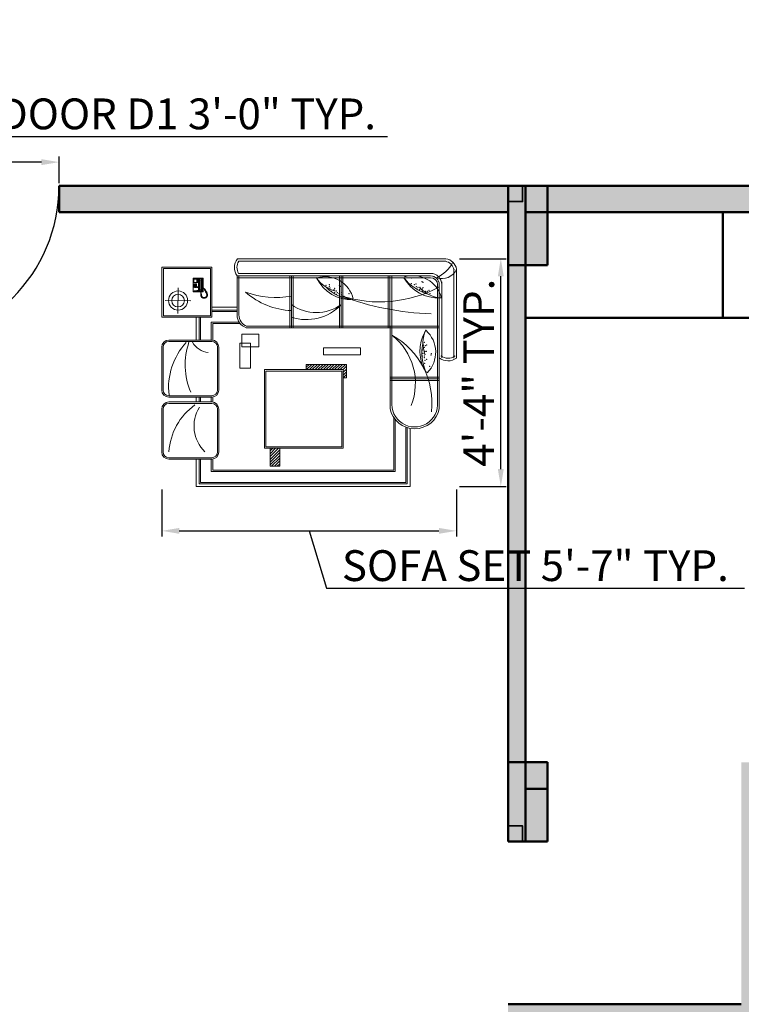
# Model space of a CAD drawing. Units: inches. Extents: x -7 to 1228, y -146 to 1091.
# Tile 24 of 88: x 269 to 433, y 307 to 531. Entities that reach past the tile are written whole.
import ezdxf

# ---------------------------------------------------------------- set-up
doc = ezdxf.new("R2010")
doc.units = ezdxf.units.IN
for name, color, linetype, lineweight in [('A-ANNO-DIMS', 2, 'Continuous', 18), ('A-COLS', 6, 'Continuous', 35), ('A-DOOR', 4, 'Continuous', 25), ('A-FURN', 8, 'Continuous', 18), ('A-WALL', 7, 'Continuous', 50), ('A-WALL-PATT', 251, 'Continuous', 13)]:
    doc.layers.add(name, color=color, linetype=linetype, lineweight=lineweight)
doc.styles.get("Standard").update_dxf_attribs({"font": 'arial.ttf'})
doc.dimstyles.new('ISO-25', dxfattribs={"dimtxt": 7, "dimasz": 4, "dimexe": 1.25, "dimexo": 0.625, "dimtad": 1, "dimdec": 1, "dimlunit": 3, "dimtxsty": 'Standard', "dimcen": 2.5, "dimadec": 0, "dimazin": 0, "dimtfac": 1, "dimtdec": 1, "dimtmove": 1, "dimatfit": 3, "dimfxl": 1, "dimarcsym": 0})

# ---------------------------------------------------------------- blocks, each defined once
blk = doc.blocks.new('A$C327A19D4')
for p, q in [((1059, 3191), (3976, 3191)), ((703, 3073), (3, 3073)), ((3, 3073), (3, 2373)), ((683, 3053), (23, 3053)), ((23, 3053), (23, 2393)), ((683, 2393), (683, 3053)), ((703, 2373), (703, 3073)), ((1078, 3155), (3976, 3155)), ((4090, 3043), (4090, 1800)), ((4126, 3043), (4126, 1800)), ((1056, 2949), (3763, 2949)), ((1056, 2403), (1056, 2949)), ((1056, 2925), (3763, 2925)), ((1076, 2985), (3780, 2985)), ((1080, 2403), (1080, 2949)), ((1791, 2223), (1791, 2949)), ((1815, 2465), (1815, 2949)), ((1839, 2223), (1839, 2949)), ((2487, 2223), (2487, 2949)), ((2511, 2223), (2511, 2949)), ((2535, 2223), (2535, 2949)), ((3169, 2223), (3169, 2949)), ((3193, 2465), (3193, 2949)), ((3221, 1195), (3221, 2949)), ((231, 2784), (227, 2425)), ((1815, 2223), (1815, 2872)), ((1815, 2223), (1815, 2872)), ((1815, 2465), (1815, 2872)), ((1815, 2465), (1815, 2872)), ((3193, 2223), (3193, 2872)), ((3193, 2223), (3193, 2872)), ((3193, 2465), (3193, 2872)), ((3193, 2465), (3193, 2872)), ((3860, 2828), (3860, 1185)), ((3884, 2828), (3884, 1095)), ((3920, 2867), (3920, 1802)), ((49, 2607), (409, 2603)), ((703, 2512), (1056, 2512)), ((3, 2373), (703, 2373)), ((23, 2393), (683, 2393)), ((484, 2052), (484, 2373)), ((524, 2052), (524, 2373)), ((544, 2052), (544, 2373)), ((703, 2472), (1056, 2472)), ((703, 2452), (1056, 2452)), ((694, 2052), (694, 2302)), ((694, 2302), (1084, 2302)), ((714, 2051), (714, 2282)), ((714, 2282), (1098, 2282)), ((3884, 2247), (1184, 2247)), ((3884, 2223), (1184, 2223)), ((3195, 2235), (3195, 1095)), ((1119, 2135), (1357, 2135)), ((1119, 1958), (1119, 2135)), ((1357, 2135), (1357, 1958)), ((1092, 2007), (1244, 2007)), ((1092, 1659), (1092, 2007)), ((1357, 1958), (1119, 1958)), ((1244, 2007), (1244, 1659)), ((2265, 1945), (2780, 1945)), ((2265, 1845), (2265, 1945)), ((2780, 1945), (2780, 1845)), ((2780, 1845), (2265, 1845)), ((1244, 1659), (1092, 1659)), ((2023, 1638), (2023, 1711)), ((2023, 1711), (2585, 1711)), ((2585, 1711), (2585, 1522)), ((2539, 1638), (1439, 1638)), ((1439, 1638), (1439, 538)), ((2519, 1618), (1459, 1618)), ((1459, 1618), (1459, 558)), ((2519, 558), (2519, 1618)), ((2539, 538), (2539, 1638)), ((2585, 1522), (2539, 1522)), ((3884, 1532), (3195, 1532)), ((3884, 1508), (3195, 1508)), ((3884, 1484), (3195, 1484)), ((484, 1185), (484, 1252)), ((524, 1185), (524, 1252)), ((544, 1185), (544, 1252)), ((694, 1185), (694, 1252)), ((714, 1184), (714, 1253)), ((3247, 967), (3247, 230)), ((3267, 940), (3267, 210)), ((3417, 832), (3417, 60)), ((3437, 825), (3437, 40)), ((3477, 816), (3477, 0)), ((1459, 558), (2519, 558)), ((1439, 538), (2539, 538)), ((1516, 538), (1651, 538)), ((1516, 285), (1516, 538)), ((1651, 538), (1651, 285)), ((484, 0), (484, 385)), ((524, 40), (524, 385)), ((544, 60), (544, 385)), ((694, 210), (694, 385)), ((714, 230), (714, 386)), ((1651, 285), (1516, 285)), ((3267, 210), (694, 210)), ((3247, 230), (714, 230)), ((3437, 40), (524, 40)), ((3417, 60), (544, 60)), ((3477, 0), (484, 0))]:
    blk.add_line(p, q)
at = {"linetype": 'ByBlock'}
for p, q in [((438, 2915), (440, 2918)), ((439, 2728), (438, 2915)), ((440, 2918), (576, 2919)), ((451, 2906), (490, 2906)), ((451, 2856), (451, 2906)), ((490, 2906), (491, 2856)), ((505, 2903), (494, 2903)), ((494, 2903), (494, 2899)), ((494, 2899), (505, 2899)), ((495, 2895), (495, 2891)), ((505, 2895), (495, 2895)), ((505, 2899), (505, 2903)), ((505, 2891), (505, 2895)), ((515, 2908), (520, 2914)), ((516, 2744), (515, 2908)), ((520, 2910), (519, 2905)), ((519, 2905), (531, 2893)), ((519, 2905), (519, 2868)), ((520, 2914), (561, 2915)), ((526, 2913), (520, 2910)), ((532, 2895), (526, 2913)), ((526, 2913), (558, 2913)), ((531, 2893), (532, 2895)), ((551, 2896), (532, 2895)), ((551, 2896), (558, 2913)), ((553, 2893), (551, 2896)), ((565, 2905), (553, 2893)), ((558, 2913), (563, 2911)), ((561, 2915), (568, 2908)), ((563, 2911), (565, 2905)), ((565, 2905), (565, 2869)), ((568, 2908), (569, 2745)), ((576, 2919), (578, 2916)), ((578, 2916), (580, 2729)), ((491, 2856), (451, 2856)), ((453, 2831), (453, 2839)), ((453, 2839), (461, 2839)), ((461, 2831), (453, 2831)), ((453, 2824), (461, 2825)), ((453, 2816), (453, 2824)), ((461, 2816), (453, 2816)), ((453, 2801), (453, 2810)), ((453, 2810), (461, 2810)), ((461, 2802), (453, 2801)), ((453, 2787), (453, 2795)), ((453, 2795), (461, 2795)), ((461, 2787), (453, 2787)), ((461, 2839), (461, 2831)), ((461, 2825), (461, 2816)), ((461, 2810), (461, 2802)), ((461, 2795), (461, 2787)), ((466, 2839), (475, 2840)), ((467, 2831), (466, 2839)), ((475, 2831), (467, 2831)), ((467, 2816), (467, 2825)), ((467, 2825), (475, 2825)), ((475, 2817), (467, 2816)), ((467, 2802), (467, 2810)), ((467, 2810), (475, 2810)), ((475, 2802), (467, 2802)), ((467, 2787), (467, 2795)), ((467, 2795), (475, 2795)), ((475, 2787), (467, 2787)), ((475, 2840), (475, 2831)), ((475, 2825), (475, 2817)), ((475, 2810), (475, 2802)), ((475, 2795), (475, 2787)), ((480, 2840), (488, 2840)), ((480, 2831), (480, 2840)), ((488, 2832), (480, 2831)), ((480, 2817), (480, 2825)), ((480, 2825), (488, 2825)), ((488, 2817), (480, 2817)), ((480, 2810), (488, 2810)), ((480, 2802), (480, 2810)), ((488, 2802), (480, 2802)), ((480, 2787), (480, 2795)), ((480, 2795), (488, 2795)), ((488, 2787), (480, 2787)), ((488, 2840), (488, 2832)), ((488, 2825), (488, 2817)), ((488, 2810), (488, 2802)), ((488, 2795), (488, 2787)), ((495, 2891), (505, 2891)), ((495, 2887), (495, 2883)), ((505, 2887), (495, 2887)), ((495, 2883), (505, 2883)), ((495, 2879), (495, 2875)), ((505, 2879), (495, 2879)), ((495, 2875), (505, 2875)), ((495, 2871), (495, 2867)), ((506, 2871), (495, 2871)), ((495, 2867), (506, 2867)), ((495, 2863), (495, 2859)), ((506, 2863), (495, 2863)), ((495, 2859), (506, 2859)), ((497, 2795), (507, 2795)), ((497, 2787), (497, 2795)), ((507, 2787), (497, 2787)), ((505, 2883), (505, 2887)), ((505, 2875), (505, 2879)), ((506, 2867), (506, 2871)), ((506, 2859), (506, 2863)), ((507, 2795), (507, 2787)), ((519, 2868), (522, 2862)), ((520, 2783), (522, 2790)), ((520, 2746), (520, 2783)), ((520, 2746), (532, 2759)), ((522, 2862), (526, 2855)), ((522, 2790), (526, 2797)), ((526, 2855), (527, 2845)), ((526, 2797), (528, 2806)), ((527, 2845), (527, 2832)), ((528, 2806), (527, 2832)), ((532, 2832), (531, 2893)), ((532, 2832), (532, 2759)), ((532, 2759), (533, 2756)), ((554, 2759), (552, 2756)), ((553, 2832), (553, 2893)), ((553, 2832), (554, 2759)), ((566, 2747), (554, 2759)), ((558, 2855), (557, 2846)), ((557, 2846), (557, 2832)), ((557, 2806), (557, 2832)), ((559, 2797), (557, 2806)), ((562, 2862), (558, 2855)), ((563, 2790), (559, 2797)), ((565, 2869), (562, 2862)), ((566, 2783), (563, 2790)), ((566, 2747), (566, 2783)), ((587, 2779), (579, 2779)), ((579, 2775), (584, 2774)), ((584, 2774), (587, 2772)), ((590, 2777), (587, 2779)), ((587, 2772), (591, 2770)), ((594, 2771), (590, 2777)), ((591, 2770), (593, 2768)), ((595, 2768), (592, 2765)), ((592, 2765), (597, 2757)), ((593, 2768), (595, 2768)), ((599, 2771), (594, 2771)), ((597, 2757), (606, 2742)), ((602, 2770), (599, 2771)), ((599, 2760), (603, 2767)), ((606, 2763), (599, 2760)), ((603, 2767), (602, 2770)), ((604, 2750), (608, 2758)), ((608, 2758), (606, 2763)), ((442, 2726), (439, 2728)), ((543, 2726), (442, 2726)), ((468, 2743), (455, 2743)), ((455, 2743), (455, 2735)), ((455, 2735), (469, 2735)), ((469, 2735), (468, 2743)), ((487, 2743), (474, 2743)), ((474, 2743), (474, 2735)), ((474, 2735), (487, 2735)), ((487, 2735), (487, 2743)), ((493, 2744), (493, 2735)), ((506, 2744), (493, 2744)), ((493, 2735), (506, 2735)), ((506, 2735), (506, 2744)), ((523, 2737), (516, 2744)), ((521, 2741), (520, 2746)), ((527, 2738), (521, 2741)), ((542, 2737), (523, 2737)), ((533, 2756), (527, 2738)), ((527, 2738), (542, 2738)), ((552, 2756), (533, 2756)), ((546, 2743), (542, 2743)), ((542, 2743), (542, 2731)), ((542, 2731), (545, 2717)), ((545, 2717), (549, 2704)), ((547, 2732), (546, 2743)), ((546, 2738), (559, 2739)), ((562, 2737), (546, 2737)), ((549, 2696), (546, 2692)), ((546, 2692), (546, 2686)), ((546, 2686), (554, 2685)), ((554, 2685), (546, 2680)), ((546, 2680), (547, 2672)), ((548, 2723), (547, 2732)), ((547, 2672), (555, 2672)), ((577, 2726), (548, 2726)), ((552, 2710), (548, 2723)), ((549, 2704), (548, 2697)), ((548, 2697), (549, 2696)), ((555, 2672), (548, 2666)), ((548, 2666), (551, 2659)), ((551, 2659), (560, 2661)), ((552, 2756), (559, 2739)), ((553, 2703), (552, 2710)), ((552, 2696), (553, 2703)), ((557, 2693), (552, 2696)), ((556, 2687), (557, 2693)), ((558, 2669), (556, 2687)), ((560, 2661), (556, 2653)), ((556, 2653), (560, 2648)), ((568, 2656), (558, 2669)), ((559, 2739), (565, 2741)), ((560, 2648), (566, 2653)), ((569, 2745), (562, 2737)), ((565, 2741), (566, 2747)), ((566, 2653), (565, 2646)), ((565, 2646), (570, 2642)), ((583, 2649), (568, 2656)), ((570, 2642), (577, 2648)), ((577, 2648), (576, 2639)), ((576, 2639), (582, 2637)), ((580, 2729), (577, 2726)), ((582, 2637), (585, 2645)), ((599, 2647), (583, 2649)), ((585, 2645), (589, 2637)), ((589, 2637), (593, 2637)), ((593, 2637), (595, 2645)), ((595, 2645), (598, 2636)), ((598, 2636), (604, 2637)), ((615, 2654), (599, 2647)), ((612, 2753), (604, 2750)), ((604, 2645), (610, 2639)), ((604, 2637), (604, 2645)), ((606, 2742), (612, 2731)), ((608, 2742), (614, 2749)), ((615, 2746), (608, 2742)), ((610, 2639), (615, 2642)), ((614, 2749), (612, 2753)), ((612, 2731), (614, 2730)), ((613, 2733), (618, 2740)), ((621, 2736), (613, 2733)), ((614, 2730), (613, 2728)), ((613, 2728), (622, 2712)), ((614, 2650), (619, 2643)), ((615, 2642), (614, 2650)), ((618, 2740), (615, 2746)), ((627, 2666), (615, 2654)), ((619, 2643), (624, 2647)), ((620, 2723), (624, 2730)), ((627, 2725), (620, 2723)), ((620, 2654), (628, 2651)), ((624, 2647), (620, 2654)), ((624, 2730), (621, 2736)), ((622, 2712), (631, 2687)), ((626, 2712), (630, 2720)), ((634, 2713), (626, 2712)), ((630, 2720), (627, 2725)), ((631, 2687), (627, 2666)), ((628, 2702), (636, 2705)), ((637, 2702), (628, 2702)), ((628, 2661), (636, 2659)), ((632, 2654), (628, 2661)), ((628, 2651), (632, 2654)), ((631, 2672), (640, 2672)), ((638, 2665), (631, 2672)), ((633, 2691), (639, 2696)), ((641, 2691), (633, 2691)), ((636, 2705), (634, 2713)), ((634, 2681), (642, 2684)), ((641, 2677), (634, 2681)), ((636, 2659), (638, 2665)), ((639, 2696), (637, 2702)), ((640, 2672), (641, 2677)), ((642, 2684), (641, 2691))]:
    blk.add_line(p, q, dxfattribs=at)
at = {"ltscale": 5}
for p, q in [((0, 1352), (0, 1952)), ((20, 1352), (20, 1952)), ((100, 2052), (700, 2052)), ((100, 2032), (700, 2032)), ((780, 1952), (780, 1352)), ((800, 1952), (800, 1352)), ((2023, 1673), (2061, 1711)), ((2027, 1638), (2100, 1711)), ((2067, 1638), (2139, 1711)), ((2106, 1638), (2179, 1711)), ((2145, 1638), (2218, 1711)), ((2184, 1638), (2257, 1711)), ((2224, 1638), (2296, 1711)), ((2263, 1638), (2336, 1711)), ((2302, 1638), (2375, 1711)), ((2341, 1638), (2414, 1711)), ((2381, 1638), (2453, 1711)), ((2420, 1638), (2493, 1711)), ((2459, 1638), (2532, 1711)), ((2498, 1638), (2571, 1711)), ((2538, 1638), (2585, 1685)), ((2539, 1601), (2585, 1646)), ((2539, 1561), (2585, 1607)), ((2539, 1522), (2585, 1568)), ((2578, 1522), (2585, 1528)), ((700, 1272), (100, 1272)), ((700, 1252), (100, 1252)), ((100, 1185), (700, 1185)), ((100, 1165), (700, 1165)), ((0, 485), (0, 1085)), ((20, 485), (20, 1085)), ((780, 1085), (780, 485)), ((800, 1085), (800, 485)), ((1516, 499), (1555, 538)), ((1516, 460), (1594, 538)), ((1516, 421), (1634, 538)), ((1516, 382), (1651, 516)), ((1516, 342), (1651, 477)), ((1516, 303), (1651, 438)), ((700, 405), (100, 405)), ((700, 385), (100, 385)), ((1537, 285), (1651, 398)), ((1576, 285), (1651, 359)), ((1616, 285), (1651, 320))]:
    blk.add_line(p, q, dxfattribs=at)
for radius in [134, 88.7]:
    blk.add_circle((229, 2605), radius)
for centre, radius, start, end in [((1218, 3068), 201, 142.4201, 216.3682), ((3943, 3007), 187, 10.9855, 79.893), ((1218, 3068), 165, 148.4003, 210.2229), ((3657, 3353), 468, 293.6733, 332.9672), ((3921, 3138), 226, 250.4844, 335.1673), ((3943, 3007), 150, 10.9855, 79.893), ((2545, 3192), 468, 214.7097, 257.8799), ((2283, 2531), 409, 13.4523, 105.9639), ((2657, 3163), 547, 207.1715, 271.8037), ((3869, 3188), 547, 208.8478, 273.48), ((3911, 3323), 657, 217.6007, 253.5739), ((3517, 2544), 409, 14.6876, 107.1992), ((3763, 2828), 157, 0, 90), ((3763, 2828), 121, 0, 90), ((3763, 2828), 96.8, 0, 90), ((2752, 3267), 657, 227.0776, 263.0508), ((3052, 4350), 1764, 252.1519, 298.1592), ((3951, 3106), 468, 222.7716, 265.9418), ((1594, 3859), 1211, 249.7283, 280.5443), ((1853, 3485), 1021, 228.2765, 267.8541), ((3865, 6197), 3777, 248.9971, 268.5461), ((2024, 3008), 670, 251.8392, 316.629), ((2163, 3036), 599, 234.5154, 305.4846), ((1243, 2401), 187, 179.2584, 251.6848), ((1243, 2401), 163, 179.2584, 251.6848), ((4159, 1898), 547, 149.1529, 213.7851), ((4124, 2008), 468, 156.691, 199.8613), ((3425, 1881), 409, 315.4337, 47.9453), ((4298, 1873), 657, 169.059, 205.0321), ((4007, 1962), 201, 232.4201, 306.3682), ((4007, 1962), 165, 232.4201, 306.3682)]:
    blk.add_arc(centre, radius, start, end)
at = {"ltscale": 20}
for centre, radius, start, end in [((2701, 1449), 849, 338.2682, 52.2695), ((2703, 1175), 1078, 353.1988, 61.2564), ((3540, 1156), 321, 172.9078, 5.2194), ((3540, 1161), 351, 190.8398, 349.1602)]:
    blk.add_arc(centre, radius, start, end, dxfattribs=at)
at = {"ltscale": 5}
for centre, radius, start, end in [((100, 1952), 100, 90, 180), ((100, 1952), 80, 90, 180), ((1024, 1388), 928, 137.1341, 186.5635), ((1307, 1706), 979, 160.9364, 203.1944), ((676, 2156), 279, 209.1633, 264.4137), ((700, 1952), 100, 0, 90), ((700, 1952), 80, 0, 90), ((100, 1352), 100, 180, 270), ((100, 1352), 80, 180, 270), ((700, 1352), 80, 270, 0), ((700, 1352), 100, 270, 0), ((100, 1085), 100, 90, 180), ((100, 1085), 80, 90, 180), ((968, 436), 868, 125.4807, 176.5616), ((949, 846), 497, 147.8484, 226.1244), ((700, 1085), 100, 0, 90), ((700, 1085), 80, 0, 90), ((100, 485), 100, 180, 270), ((100, 485), 80, 180, 270), ((700, 485), 100, 270, 0), ((700, 485), 80, 270, 0)]:
    blk.add_arc(centre, radius, start, end, dxfattribs=at)
for p in [(3492, 2920), (2298, 2818), (2329, 2780), (2344, 2802), (2345, 2825), (2356, 2781), (2410, 2757), (2421, 2774), (2485, 2814), (2498, 2803), (3495, 2842), (3535, 2825), (3560, 2838), (3561, 2800), (3571, 2765), (3585, 2789), (3609, 2758), (3612, 2788), (3641, 2868), (3647, 2768), (3655, 2787), (3657, 2862), (2375, 2736), (2421, 2720), (2444, 2738), (2445, 2691), (2459, 2715), (2481, 2700), (2514, 2718), (2515, 2690), (2551, 2664), (2620, 2701), (3646, 2728), (3694, 2735), (3707, 2710), (3719, 2734), (3738, 2747), (3756, 2703), (3660, 1974), (3676, 1951), (3677, 2020), (3687, 1973), (3707, 1984), (3646, 1828), (3648, 1911), (3658, 1864), (3673, 1803), (3674, 1829), (3684, 1893), (3686, 1853), (3705, 1892), (3770, 1842), (3772, 1859), (3680, 1724), (3683, 1768), (3706, 1784), (3748, 1685)]:
    blk.add_point(p)
blk = doc.blocks.new('DOOR-900')
blk.add_line((36, 0), (36, 36))
blk.add_arc((36, 0), 36, 90, 180)
blk = doc.blocks.new('*D40')
at = {"layer": 'A-ANNO-DIMS', "color": 0, "lineweight": -2, "transparency": 16777216}
for p, q in [((301.32, 424.02), (301.32, 413.35)), ((368.31, 424.02), (368.31, 413.35)), ((305.32, 414.6), (364.31, 414.6)), ((334.82, 414.6), (338.73, 401.55)), ((338.73, 401.55), (433.69, 401.55))]:
    blk.add_line(p, q, dxfattribs=at)
at = {"layer": 'A-ANNO-DIMS', "color": 0, "transparency": 16777216}
for points in [[(305.32, 415.26), (305.32, 413.93), (301.32, 414.6)], [(364.31, 415.26), (364.31, 413.93), (368.31, 414.6)]]:
    blk.add_solid(points, dxfattribs=at)
at = {"layer": 'Defpoints', "color": 0, "transparency": 16777216}
for p in [(301.32, 424.65), (368.31, 424.65), (368.31, 414.6)]:
    blk.add_point(p, dxfattribs=at)
at = {"layer": 'A-ANNO-DIMS', "color": 0, "transparency": 16777216, "insert": (386.21, 405.79), "char_height": 7, "attachment_point": 5}
blk.add_mtext('SOFA SET 5\'-7" TYP.', dxfattribs=at)
blk = doc.blocks.new('*D41')
at = {"layer": 'A-ANNO-DIMS', "color": 0, "lineweight": -2, "transparency": 16777216}
for p, q in [((368.94, 476.46), (379.61, 476.46)), ((378.36, 428.65), (378.36, 472.46)), ((368.94, 424.65), (379.61, 424.65))]:
    blk.add_line(p, q, dxfattribs=at)
at = {"layer": 'A-ANNO-DIMS', "color": 0, "transparency": 16777216}
for points in [[(377.69, 472.46), (379.03, 472.46), (378.36, 476.46)], [(377.69, 428.65), (379.03, 428.65), (378.36, 424.65)]]:
    blk.add_solid(points, dxfattribs=at)
at = {"layer": 'Defpoints', "color": 0, "transparency": 16777216}
for p in [(368.31, 476.46), (378.36, 476.46), (368.31, 424.65)]:
    blk.add_point(p, dxfattribs=at)
at = {"layer": 'A-ANNO-DIMS', "color": 0, "transparency": 16777216, "insert": (374.23, 450.55), "char_height": 7, "attachment_point": 5, "rotation": 90}
blk.add_mtext('4\'-4" TYP.', dxfattribs=at)
blk = doc.blocks.new('*D44')
at = {"layer": 'A-ANNO-DIMS', "color": 0, "lineweight": -2, "transparency": 16777216}
for p, q in [((260, 498.4), (261.74, 504.21)), ((261.74, 504.21), (352.58, 504.21)), ((242, 493.62), (242, 499.65)), ((278, 493.62), (278, 499.65)), ((274, 498.4), (246, 498.4))]:
    blk.add_line(p, q, dxfattribs=at)
at = {"layer": 'A-ANNO-DIMS', "color": 0, "transparency": 16777216}
for points in [[(246, 499.07), (246, 497.73), (242, 498.4)], [(274, 499.07), (274, 497.73), (278, 498.4)]]:
    blk.add_solid(points, dxfattribs=at)
at = {"layer": 'Defpoints', "color": 0, "transparency": 16777216}
for p in [(242, 498.4), (242, 493), (278, 493)]:
    blk.add_point(p, dxfattribs=at)
at = {"layer": 'A-ANNO-DIMS', "color": 0, "transparency": 16777216, "insert": (307.16, 508.46), "char_height": 7, "attachment_point": 5}
blk.add_mtext('DOOR D1 3\'-0" TYP.', dxfattribs=at)

msp = doc.modelspace()

# ---------------------------------------------------------------- hatches: boundary and pattern name
at = {"layer": 'A-COLS'}
h = msp.add_hatch(color=256, dxfattribs=at)
h.dxf.hatch_style = 1
h.paths.add_polyline_path([(380, 475), (389, 475), (389, 493), (383.29, 493), (383.29, 489.45), (380, 489.45)])
h = msp.add_hatch(color=256, dxfattribs=at)
h.dxf.hatch_style = 1
h.paths.add_polyline_path([(383.29, 489.45), (383.29, 493), (380, 493), (380, 489.45)])
h = msp.add_hatch(color=256, dxfattribs=at)
h.dxf.hatch_style = 1
h.paths.add_polyline_path([(380, 347.55), (383.29, 347.55), (383.29, 344), (389, 344), (389, 362), (380, 362)])
h = msp.add_hatch(color=256, dxfattribs=at)
h.dxf.hatch_style = 1
h.paths.add_polyline_path([(380, 347.55), (380, 344), (383.29, 344), (383.29, 347.55)])
at = {"layer": 'A-WALL-PATT'}
h = msp.add_hatch(color=256, dxfattribs=at)
h.dxf.hatch_style = 1
h.paths.add_polyline_path([(69, 568), (60, 568), (60, 493), (63.29, 493), (69, 493)])
h.paths.add_polyline_path([(69, 662.41), (60, 662.41), (60, 586), (69, 586)], flags=17)
h.paths.add_polyline_path([(69, 723), (184, 723), (184, 734), (179, 734), (179, 728), (69, 728), (69, 741.62), (60, 741.62), (60, 698.41), (69, 698.41)], flags=17)
h.paths.add_polyline_path([(69, 782), (231, 782), (231, 728), (231, 723), (231, 586), (236, 586), (236, 787), (69, 787), (69, 800.13), (60, 800.13), (60, 765.62), (69, 765.62)])
h.paths.add_polyline_path([(184, 842), (189, 842), (189, 848), (173, 848), (173, 842), (179, 842), (179, 787), (184, 787)])
h.paths.add_polyline_path([(118.22, 69), (69, 69), (69, 60), (118.22, 60)])
h.paths.add_polyline_path([(227, 69), (154.22, 69), (154.22, 60), (227, 60)])
h.paths.add_polyline_path([(236, 60), (232.71, 60), (227, 60), (227, 36), (236, 36)])
h.paths.add_polyline_path([(389, 60), (380, 60), (380, 36), (389, 36)])
h.paths.add_polyline_path([(384, 181), (380, 181), (380, 115), (380, 78), (384, 78)])
h.paths.add_polyline_path([(380, 115), (334.55, 115), (334.55, 109), (380, 109)])
h.paths.add_polyline_path([(274.55, 115), (236, 115), (236, 201), (232.71, 201), (231, 201), (231, 78), (236, 78), (236, 109), (274.55, 109)])
h.paths.add_polyline_path([(69, 123), (60, 123), (60, 78), (69, 78)])
h.paths.add_polyline_path([(69, 201), (60, 201), (60, 159), (69, 159)])
h.paths.add_polyline_path([(143, 219), (69, 219), (69, 213), (143, 213)], flags=17)
h.paths.add_polyline_path([(189, 219), (184, 219), (184, 274), (231, 274), (231, 219), (236, 219), (236, 279), (184, 279), (184, 297), (179, 297), (179, 279), (69, 279), (69, 290.91), (60, 290.91), (60, 262.18), (69, 262.18), (69, 274), (179, 274), (179, 219), (173, 219), (173, 213), (189, 213)])
h.paths.add_polyline_path([(69, 238.18), (60, 238.18), (60, 219), (69, 219)], flags=17)
h.paths.add_polyline_path([(69, 333), (60, 333), (60, 314.91), (69, 314.91), (69, 316.96)])
h.paths.add_polyline_path([(190, 338), (184, 338), (69, 338), (69, 333), (179, 333), (179, 327), (184, 327), (184, 333.02), (190, 333.05)])
h.paths.add_polyline_path([(69, 386.81), (60, 386.81), (60, 351), (69, 351)])
h.paths.add_polyline_path([(69, 475), (60, 475), (60, 422.81), (69, 422.81)])
h.paths.add_polyline_path([(236, 475), (231, 475), (231, 351.24), (236, 351.24)])
h.paths.add_polyline_path([(384, 475), (380, 475), (380, 362), (384, 362)])
h.paths.add_polyline_path([(547, 307), (439, 307), (439, 356), (445, 356), (445, 362), (433, 362), (433, 307), (380, 307), (380, 244), (380, 241), (384, 241), (384, 301), (433, 301), (433, 277), (439, 277), (439, 301), (547, 301)])
h.paths.add_polyline_path([(547, 241), (439, 241), (439, 247), (433, 247), (433, 235), (547, 235)])
h.paths.add_polyline_path([(450, 69), (440.29, 69), (424.89, 69), (389, 69), (389, 60), (450, 60)])
h.paths.add_polyline_path([(547, 69), (486, 69), (486, 60), (547, 60)])
h.paths.add_polyline_path([(556, 148.27), (547, 148.27), (547, 78), (556, 78)])
h.paths.add_polyline_path([(556, 223), (547, 223), (547, 195), (547, 184.27), (556, 184.27)])
h.paths.add_polyline_path([(556, 311.19), (547, 311.19), (547, 273.08), (556, 273.08)])
h.paths.add_polyline_path([(556, 344), (552.71, 344), (547, 344), (547, 335.19), (556, 335.19)])
h.paths.add_polyline_path([(556, 249.08), (547, 249.08), (547, 241), (556, 241)])
h.paths.add_polyline_path([(547, 362), (475, 362), (475, 356), (547, 356)], flags=0)
h.paths.add_polyline_path([(556, 399.62), (547, 399.62), (547, 362), (556, 362)])
h.paths.add_polyline_path([(556, 475), (547, 475), (547, 435.62), (556, 435.62)])
h.paths.add_polyline_path([(547, 493), (389, 493), (389, 487), (547, 487)])
h.paths.add_polyline_path([(380, 493), (278, 493), (278, 487), (380, 487)])
h.paths.add_polyline_path([(227, 493), (69, 493), (69, 487), (227, 487)])
h.paths.add_polyline_path([(643, 122.44), (634, 122.44), (634, 78), (643, 78)])
h.paths.add_polyline_path([(702.5, 69), (692.79, 69), (677.39, 69), (643, 69), (643, 60), (702.5, 60)])
h.paths.add_polyline_path([(798, 69), (738.5, 69), (738.5, 60), (798, 60)])
h.paths.add_polyline_path([(807, 60), (803.71, 60), (798, 60), (798, 36), (807, 36)])
h.paths.add_polyline_path([(807, 109), (846.75, 109), (846.75, 115), (807, 115), (807, 159), (802, 159), (802, 78), (807, 78)])
h.paths.add_polyline_path([(807, 201), (802, 201), (802, 195), (807, 195)])
h.paths.add_polyline_path([(643, 201), (634, 201), (634, 158.44), (643, 158.44)])
h.paths.add_polyline_path([(756, 225), (751, 225), (751, 219), (643, 219), (643, 213), (756, 213)])
h.paths.add_polyline_path([(643, 240.85), (634, 240.85), (634, 219), (643, 219)])
h.paths.add_polyline_path([(643, 274), (643, 288.63), (634, 288.63), (634, 264.85), (643, 264.85)])
h.paths.add_polyline_path([(802, 279), (756, 279), (756, 297), (751, 297), (751, 279), (643, 279), (643, 274), (751, 274), (751, 255), (756, 255), (756, 274), (802, 274)])
h.paths.add_polyline_path([(807, 333), (803.71, 333), (802, 333), (802, 279), (802, 274), (802, 219), (807, 219)])
h.paths.add_polyline_path([(956, 182), (951, 182), (951, 115), (906.75, 115), (906.75, 109), (951, 109), (951, 78), (956, 78)])
h.paths.add_polyline_path([(960, 60), (951, 60), (951, 36), (960, 36)])
h.paths.add_polyline_path([(1021, 69), (1005.78, 69), (960, 69), (960, 60), (1021, 60)])
h.paths.add_polyline_path([(956, 224), (951, 224), (951, 218), (956, 218)])
h.paths.add_polyline_path([(956, 302), (1004, 302), (1004, 278), (1010, 278), (1010, 302), (1118, 302), (1118, 290.81), (1127, 290.81), (1127, 326.97), (1118, 326.97), (1118, 320.97), (1118, 307), (1010, 307), (1010, 356), (1016, 356), (1016, 362), (1004, 362), (1004, 307), (951, 307), (951, 244), (951, 242), (954.29, 242), (956, 242)])
h.paths.add_polyline_path([(643, 333), (634, 333), (634, 312.63), (643, 312.63), (643, 316.96)])
h.paths.add_polyline_path([(756, 338), (643, 338), (643, 333), (751, 333), (751, 327), (756, 327)])
h.paths.add_polyline_path([(643, 388), (634, 388), (634, 351), (643, 351)])
h.paths.add_polyline_path([(807, 357), (802, 357), (802, 351), (807, 351)])
h.paths.add_polyline_path([(807, 475), (802, 475), (802, 393), (807, 393)])
h.paths.add_polyline_path([(643, 475), (634, 475), (634, 424), (643, 424)])
h.paths.add_polyline_path([(798, 493), (643, 493), (643, 487), (798, 487)])
h.paths.add_polyline_path([(634, 493), (556, 493), (556, 487), (634, 487)])
h.paths.add_polyline_path([(813, 493), (807, 493), (807, 487), (813, 487)])
h.paths.add_polyline_path([(951, 493), (849, 493), (849, 487), (951, 487)])
h.paths.add_polyline_path([(956, 484), (951, 484), (951, 374), (956, 374)])
h.paths.add_polyline_path([(1109, 493), (969, 493), (969, 487), (1109, 487)])
h.paths.add_polyline_path([(1127, 484), (1118, 484), (1118, 450.64), (1127, 450.64)])
h.paths.add_polyline_path([(1127, 414.64), (1118, 414.64), (1118, 365), (1127, 365)])
h.paths.add_polyline_path([(1109, 362), (1046, 362), (1046, 356), (1109, 356)], flags=17)
h.paths.add_polyline_path([(1127, 356), (1123.45, 356), (1118, 356), (1118, 350.97), (1127, 350.97)], flags=0)
h.paths.add_polyline_path([(1127, 266.81), (1118, 266.81), (1118, 262.36), (1118, 242), (1127, 242)], flags=17)
h.paths.add_polyline_path([(1118, 242), (1010, 242), (1010, 248), (1004, 248), (1004, 237), (1118, 237)])
h.paths.add_polyline_path([(1127, 224), (1118, 224), (1118, 170), (1127, 170)])
h.paths.add_polyline_path([(1127, 134), (1118, 134), (1118, 78), (1127, 78)])
h.paths.add_polyline_path([(1118, 69), (1057, 69), (1057, 60), (1118, 60)])
h.paths.add_polyline_path([(227, 571.55), (227, 574), (69, 574), (69, 568), (227, 568)])
h.paths.add_polyline_path([(380, 571.55), (380, 574), (278, 574), (278, 568), (380, 568)])
h.paths.add_polyline_path([(242, 574), (236, 574), (236, 568), (242, 568)])
h.paths.add_polyline_path([(547, 571.55), (547, 574), (389, 574), (389, 568), (547, 568)])
h.paths.add_polyline_path([(384, 733), (380, 733), (380, 586), (384, 586)])
h.paths.add_polyline_path([(556, 646), (634, 646), (634, 655), (547, 655), (547, 586), (556, 586)])
h.paths.add_polyline_path([(634, 574), (556, 574), (556, 568), (634, 568)])
h.paths.add_polyline_path([(643, 655), (634, 655), (634, 586), (643, 586)])
h.paths.add_polyline_path([(798, 574), (643, 574), (643, 568), (798, 568)])
h.paths.add_polyline_path([(643, 663.85), (634, 663.85), (634, 655), (643, 655)])
h.paths.add_polyline_path([(556, 676.97), (547, 676.97), (547, 655), (556, 655)])
h.paths.add_polyline_path([(556, 733), (547, 733), (547, 712.97), (556, 712.97)])
h.paths.add_polyline_path([(643, 710), (634, 710), (634, 699.85), (643, 699.85)])
h.paths.add_polyline_path([(807, 668), (802, 668), (802, 586), (807, 586)])
h.paths.add_polyline_path([(951, 574), (849, 574), (849, 568), (951, 568)])
h.paths.add_polyline_path([(956, 691), (951, 691), (951, 577), (956, 577)])
h.paths.add_polyline_path([(1109, 574), (969, 574), (969, 568), (1109, 568)])
h.paths.add_polyline_path([(1127, 643.4), (1118, 643.4), (1118, 577), (1127, 577)])
h.paths.add_polyline_path([(1127, 568), (1123.45, 568), (1118, 568), (1118, 493), (1127, 493)])
h.paths.add_polyline_path([(1127, 733), (1118, 733), (1118, 679.4), (1127, 679.4)])
h.paths.add_polyline_path([(1127, 777.35), (1118, 777.35), (1118, 770.04), (1118, 751), (1127, 751)], flags=17)
h.paths.add_polyline_path([(1118, 751), (1010, 751), (1010, 757), (1004, 757), (1004, 745), (1118, 745)])
h.paths.add_polyline_path([(956, 811), (1004, 811), (1004, 787), (1010, 787), (1010, 811), (1017.87, 811), (1017.87, 811.63, -0.414214), (1018.25, 812), (1031.98, 812, -0.414214), (1032.35, 811.63), (1032.35, 811), (1118, 811), (1118, 801.35), (1127, 801.35), (1127, 834.69), (1118, 834.69), (1118, 830.24), (1118, 817), (1010, 817), (1010, 866), (1016, 866), (1016, 872), (1004, 872), (1004, 817), (956, 817), (956, 866), (951, 866), (951, 751), (954.29, 751), (956, 751)])
h.paths.add_polyline_path([(1118, 872), (1046, 872), (1046, 866), (1118, 866)], flags=17)
h.paths.add_polyline_path([(1127, 924.71), (1118, 924.71), (1118, 884), (1127, 884)])
h.paths.add_polyline_path([(1127, 866), (1123.71, 866), (1118, 866), (1118, 858.69), (1127, 858.69)], flags=17)
h.paths.add_polyline_path([(956, 983), (951, 983), (951, 952), (807, 952), (807, 983), (802, 983), (802, 902), (807, 902), (807, 946), (951, 946), (951, 884), (956, 884)])
h.paths.add_polyline_path([(807, 842), (802, 842), (802, 787), (756, 787), (756, 806), (751, 806), (751, 787), (643, 787), (643, 782), (751, 782), (751, 764), (756, 764), (756, 782), (802, 782), (802, 728), (807, 728)])
h.paths.add_polyline_path([(756, 848), (643, 848), (643, 842), (751, 842), (751, 836), (756, 836)])
h.paths.add_polyline_path([(756, 734), (751, 734), (751, 728), (643, 728), (643, 723), (756, 723)])
h.paths.add_polyline_path([(643, 749.79), (634, 749.79), (634, 728), (637.29, 728), (643, 728)])
h.paths.add_polyline_path([(643, 805.41), (634, 805.41), (634, 773.79), (643, 773.79)])
h.paths.add_polyline_path([(643, 896.66), (634, 896.66), (634, 860), (637.29, 860), (643, 860)])
h.paths.add_polyline_path([(643, 842), (634, 842), (634, 829.41), (643, 829.41)])
h.paths.add_polyline_path([(643, 983), (634, 983), (634, 932.66), (643, 932.66)])
h.paths.add_polyline_path([(1127, 983), (1118, 983), (1118, 960.71), (1127, 960.71)])
h.paths.add_polyline_path([(1118, 1001), (1077.53, 1001), (1077.53, 992), (1118, 992)])
h.paths.add_polyline_path([(1041.53, 1001), (960, 1001), (960, 992), (1041.53, 992)])
h.paths.add_polyline_path([(960, 1025), (951, 1025), (951, 1001), (954.29, 1001), (960, 1001)])
h.paths.add_polyline_path([(807, 1025), (798, 1025), (798, 1001), (807, 1001)])
h.paths.add_polyline_path([(798, 1001), (738.5, 1001), (738.5, 992), (798, 992)])
h.paths.add_polyline_path([(702.5, 1001), (643, 1001), (643, 992), (702.5, 992)])
h.paths.add_polyline_path([(547, 1001), (499.11, 1001), (499.11, 992), (547, 992)])
h.paths.add_polyline_path([(463.11, 1001), (389, 1001), (389, 992), (463.11, 992)])
h.paths.add_polyline_path([(389, 1025), (380, 1025), (380, 1022), (380, 1001), (383.29, 1001), (389, 1001)])
h.paths.add_polyline_path([(236, 1025), (227, 1025), (227, 1001), (236, 1001)])
h.paths.add_polyline_path([(236, 983), (231, 983), (231, 860), (236, 860)])
h.paths.add_polyline_path([(274.55, 952), (236, 952), (236, 946), (274.55, 946)])
h.paths.add_polyline_path([(380, 952), (334.55, 952), (334.55, 946), (380, 946)])
h.paths.add_polyline_path([(384, 983), (380, 983), (380, 884), (383.29, 884), (384, 884)])
h.paths.add_polyline_path([(227, 1001), (155.01, 1001), (155.01, 992), (162.87, 992), (227, 992)])
h.paths.add_polyline_path([(119.01, 1001), (69, 1001), (69, 992), (119.01, 992)])
h.paths.add_polyline_path([(69, 983), (60, 983), (60, 922.99), (69, 922.99)])
h.paths.add_polyline_path([(69, 886.99), (60, 886.99), (60, 860), (63.29, 860), (69, 860)])
h.paths.add_polyline_path([(143, 848), (69, 848), (69, 842), (143, 842)])

# ---------------------------------------------------------------- linework, layer by layer
at = {"layer": 'A-COLS'}
for points in [[(380, 493), (383.29, 493), (383.29, 489.45), (380, 489.45)], [(380, 344), (383.29, 344), (383.29, 347.55), (380, 347.55)]]:
    msp.add_lwpolyline(points, close=True, dxfattribs=at)
at = {"layer": 'A-WALL'}
for p, q in [((380, 493), (278, 493)), ((278, 487), (278, 493)), ((380, 493), (380, 344)), ((380, 493), (389, 493)), ((380, 475), (380, 493)), ((384, 493), (384, 344)), ((547, 493), (384, 493)), ((389, 493), (389, 475)), ((380, 487), (278, 487)), ((380, 344), (380, 487)), ((547, 487), (384, 487)), ((384, 344), (384, 487)), ((428.83, 463), (428.83, 487)), ((389, 475), (380, 475)), ((523, 463), (384, 463)), ((389, 362), (380, 362)), ((380, 362), (380, 344)), ((389, 362), (384, 362)), ((389, 344), (389, 362)), ((389, 362), (389, 356)), ((389, 356), (384, 356)), ((380, 344), (389, 344)), ((433, 307), (380, 307))]:
    msp.add_line(p, q, dxfattribs=at)

# ---------------------------------------------------------------- block references
at = {"layer": 'A-DOOR', "rotation": 180}
msp.add_blockref('DOOR-900', (278, 493), dxfattribs=at)
at = {"layer": 'A-FURN', "xscale": 0.016235792481004, "yscale": 0.016235792481004, "zscale": 0.016235792481004}
msp.add_blockref('A$C327A19D4', (301.32, 424.65), dxfattribs=at)

# ---------------------------------------------------------------- dimensions: what is measured, and where the dimension line sits
at = {"layer": 'A-ANNO-DIMS'}
for base, p1, p2, angle, text, picture, middle in [((242, 498.4), (278, 493), (242, 493), 180, 'DOOR D1 <> TYP.', '*D44', (262.37, 508.46)), ((378.36, 476.46), (368.31, 424.65), (368.31, 476.46), 90, '<> TYP.', '*D41', (374.23, 450.55))]:
    dim = msp.add_linear_dim(base=base, p1=p1, p2=p2, angle=angle, text=text, dimstyle='ISO-25', override={"dimdec": 1, "dimlfac": 1, "dimrnd": 0, "dimzin": 1, "dimdsep": 46, "dimlunit": 4, "dimfrac": 2}, dxfattribs=at)
    dim.commit()
    dim.dimension.update_dxf_attribs({"geometry": picture, "text_midpoint": middle})
dim = msp.add_linear_dim(base=(368.31, 414.6), p1=(301.32, 424.65), p2=(368.31, 424.65), text='SOFA SET <> TYP.', dimstyle='ISO-25', override={"dimdec": 1, "dimlfac": 1, "dimrnd": 0, "dimzin": 1, "dimdsep": 46, "dimlunit": 4, "dimfrac": 2}, dxfattribs=at)
dim.commit()
dim.dimension.update_dxf_attribs({"geometry": '*D40', "text_midpoint": (339.36, 405.79)})

doc.saveas('drawing.dxf')
